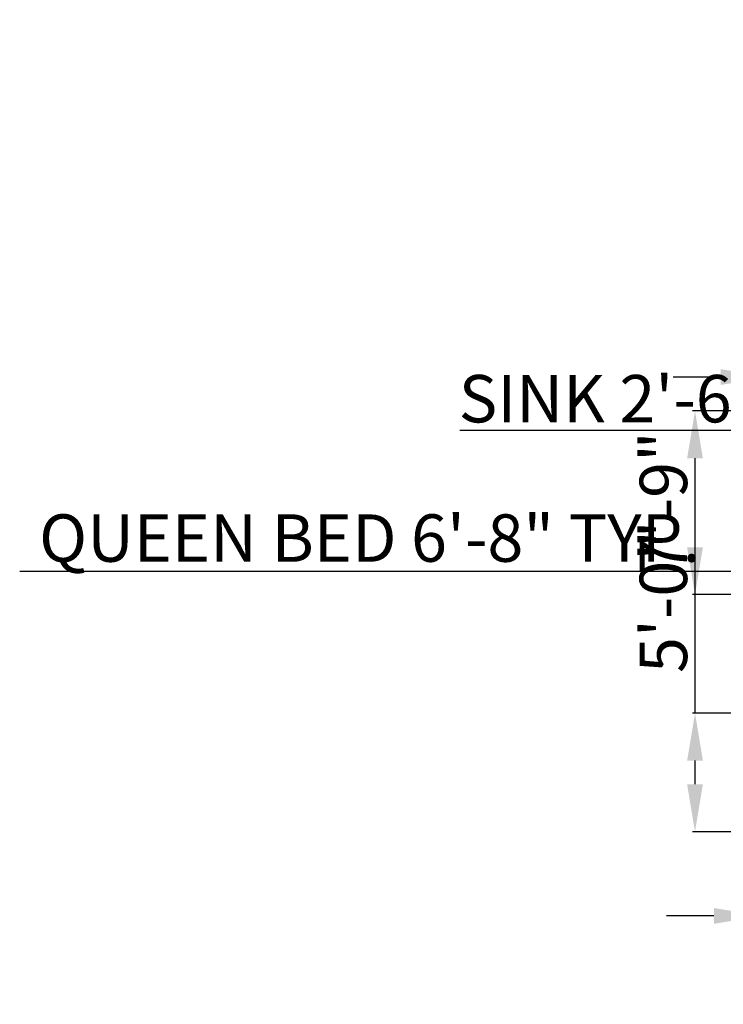
# Model space of a CAD drawing. Units: inches. Extents: x -584 to 444, y 228 to 1001.
# Tile 1 of 5: x -584 to -228, y 298 to 797. Entities that reach past the tile are written whole.
import ezdxf

# ---------------------------------------------------------------- set-up
doc = ezdxf.new("R2010")
doc.units = ezdxf.units.IN
doc.layers.add('A-ANNO-DIMS', color=2, linetype='Continuous', lineweight=18)
doc.styles.get("Standard").update_dxf_attribs({"font": 'arial.ttf'})
doc.dimstyles.new('ISO-25', dxfattribs={"dimtxt": 24, "dimasz": 24, "dimexe": 1.25, "dimexo": 0.625, "dimtad": 1, "dimdec": 1, "dimlunit": 3, "dimtxsty": 'Standard', "dimcen": 2.5, "dimadec": 0, "dimazin": 0, "dimtfac": 1, "dimtdec": 1, "dimtmove": 0, "dimatfit": 3, "dimfxl": 1, "dimarcsym": 0})

# ---------------------------------------------------------------- blocks, each defined once
blk = doc.blocks.new('*D15')
at = {"layer": 'A-ANNO-DIMS', "color": 0, "lineweight": -2, "transparency": 16777216}
for p, q in [((-206.06, 505.93), (-206.06, 518.55)), ((-126.06, 505.93), (-126.06, 518.55)), ((-206.06, 517.3), (-584.35, 517.3)), ((-150.06, 517.3), (-182.06, 517.3))]:
    blk.add_line(p, q, dxfattribs=at)
at = {"layer": 'A-ANNO-DIMS', "color": 0, "transparency": 16777216}
for points in [[(-182.06, 521.3), (-182.06, 513.3), (-206.06, 517.3)], [(-150.06, 521.3), (-150.06, 513.3), (-126.06, 517.3)]]:
    blk.add_solid(points, dxfattribs=at)
at = {"layer": 'Defpoints', "color": 0, "transparency": 16777216}
for p in [(-206.06, 517.3), (-206.06, 505.3), (-126.06, 505.3)]:
    blk.add_point(p, dxfattribs=at)
at = {"layer": 'A-ANNO-DIMS', "color": 0, "transparency": 16777216, "insert": (-407.21, 531.07), "char_height": 24, "attachment_point": 5}
blk.add_mtext('QUEEN BED 6\'-8" TYP.', dxfattribs=at)
blk = doc.blocks.new('*D19')
at = {"layer": 'A-ANNO-DIMS', "color": 0, "lineweight": -2, "transparency": 16777216}
for p, q in [((-185.21, 588.56), (-361.72, 588.56)), ((-161.21, 584.69), (-161.21, 589.81)), ((-131.21, 588.56), (-161.21, 588.56)), ((-131.21, 584.69), (-131.21, 589.81)), ((-107.21, 588.56), (-83.21, 588.56))]:
    blk.add_line(p, q, dxfattribs=at)
at = {"layer": 'A-ANNO-DIMS', "color": 0, "transparency": 16777216}
for points in [[(-185.21, 592.56), (-185.21, 584.56), (-161.21, 588.56)], [(-107.21, 592.56), (-107.21, 584.56), (-131.21, 588.56)]]:
    blk.add_solid(points, dxfattribs=at)
at = {"layer": 'Defpoints', "color": 0, "transparency": 16777216}
for p in [(-161.21, 588.56), (-161.21, 584.06), (-131.21, 584.06)]:
    blk.add_point(p, dxfattribs=at)
at = {"layer": 'A-ANNO-DIMS', "color": 0, "transparency": 16777216, "insert": (-285.47, 601.6), "char_height": 24, "attachment_point": 5}
blk.add_mtext('SINK 2\'-6"', dxfattribs=at)
blk = doc.blocks.new('*D21')
at = {"layer": 'A-ANNO-DIMS', "color": 0, "lineweight": -2, "transparency": 16777216}
for p, q in [((-186.99, 636.91), (-186.99, 660.91)), ((-189.13, 612.91), (-185.74, 612.91)), ((-186.99, 612.91), (-186.99, 594.47)), ((-189.13, 594.47), (-185.74, 594.47)), ((-186.99, 570.47), (-186.99, 298.2))]:
    blk.add_line(p, q, dxfattribs=at)
at = {"layer": 'A-ANNO-DIMS', "color": 0, "transparency": 16777216}
for points in [[(-190.99, 636.91), (-182.99, 636.91), (-186.99, 612.91)], [(-190.99, 570.47), (-182.99, 570.47), (-186.99, 594.47)]]:
    blk.add_solid(points, dxfattribs=at)
at = {"layer": 'Defpoints', "color": 0, "transparency": 16777216}
for p in [(-189.76, 612.91), (-189.76, 594.47), (-186.99, 594.47)]:
    blk.add_point(p, dxfattribs=at)
at = {"layer": 'A-ANNO-DIMS', "color": 0, "transparency": 16777216, "insert": (-200.02, 422.34), "char_height": 24, "attachment_point": 5, "rotation": 90}
blk.add_mtext('RANGE 1\'-6 1/2"', dxfattribs=at)
blk = doc.blocks.new('*D22')
at = {"layer": 'A-ANNO-DIMS', "color": 0, "lineweight": -2, "transparency": 16777216}
for p, q in [((-229.74, 615.68), (-253.74, 615.68)), ((-205.74, 613.54), (-205.74, 616.93)), ((-205.74, 615.68), (-189.76, 615.68)), ((-189.76, 613.54), (-189.76, 616.93)), ((-165.76, 615.68), (-78.97, 615.68))]:
    blk.add_line(p, q, dxfattribs=at)
at = {"layer": 'A-ANNO-DIMS', "color": 0, "transparency": 16777216}
for points in [[(-229.74, 619.68), (-229.74, 611.68), (-205.74, 615.68)], [(-165.76, 619.68), (-165.76, 611.68), (-189.76, 615.68)]]:
    blk.add_solid(points, dxfattribs=at)
at = {"layer": 'Defpoints', "color": 0, "transparency": 16777216}
for p in [(-189.76, 615.68), (-205.74, 612.91), (-189.76, 612.91)]:
    blk.add_point(p, dxfattribs=at)
at = {"layer": 'A-ANNO-DIMS', "color": 0, "transparency": 16777216, "insert": (-110.36, 628.35), "char_height": 24, "attachment_point": 5}
blk.add_mtext('1\'-4"', dxfattribs=at)
blk = doc.blocks.new('*D29')
at = {"layer": 'A-ANNO-DIMS', "color": 0, "lineweight": -2, "transparency": 16777216}
for p, q in [((-209.14, 795.91), (-209.14, 341.69)), ((-176.14, 795.91), (-176.14, 341.69)), ((-233.14, 342.94), (-257.14, 342.94)), ((-209.14, 342.94), (-176.14, 342.94)), ((-152.14, 342.94), (-62.69, 342.94))]:
    blk.add_line(p, q, dxfattribs=at)
at = {"layer": 'A-ANNO-DIMS', "color": 0, "transparency": 16777216}
for points in [[(-233.14, 346.94), (-233.14, 338.94), (-209.14, 342.94)], [(-152.14, 346.94), (-152.14, 338.94), (-176.14, 342.94)]]:
    blk.add_solid(points, dxfattribs=at)
at = {"layer": 'Defpoints', "color": 0, "transparency": 16777216}
for p in [(-209.14, 796.54), (-176.14, 796.54), (-176.14, 342.94)]:
    blk.add_point(p, dxfattribs=at)
at = {"layer": 'A-ANNO-DIMS', "color": 0, "transparency": 16777216, "insert": (-95.41, 355.82), "char_height": 24, "attachment_point": 5}
blk.add_mtext('2\'-9"', dxfattribs=at)
blk = doc.blocks.new('*D33')
at = {"layer": 'A-ANNO-DIMS', "color": 0, "lineweight": -2, "transparency": 16777216}
for p, q in [((-242.74, 445.54), (-242.74, 534.59)), ((-218.77, 445.54), (-243.99, 445.54)), ((-242.74, 409.54), (-242.74, 421.54)), ((-218.77, 385.54), (-243.99, 385.54))]:
    blk.add_line(p, q, dxfattribs=at)
at = {"layer": 'A-ANNO-DIMS', "color": 0, "transparency": 16777216}
for points in [[(-246.74, 421.54), (-238.74, 421.54), (-242.74, 445.54)], [(-246.74, 409.54), (-238.74, 409.54), (-242.74, 385.54)]]:
    blk.add_solid(points, dxfattribs=at)
at = {"layer": 'Defpoints', "color": 0, "transparency": 16777216}
for p in [(-242.74, 445.54), (-218.14, 445.54), (-218.14, 385.54)]:
    blk.add_point(p, dxfattribs=at)
at = {"layer": 'A-ANNO-DIMS', "color": 0, "transparency": 16777216, "insert": (-255.62, 502.06), "char_height": 24, "attachment_point": 5, "rotation": 90}
blk.add_mtext('5\'-0"', dxfattribs=at)
blk = doc.blocks.new('*D34')
at = {"layer": 'A-ANNO-DIMS', "color": 0, "lineweight": -2, "transparency": 16777216}
for p, q in [((-218.77, 598.54), (-243.99, 598.54)), ((-242.74, 529.54), (-242.74, 574.54)), ((-218.77, 505.54), (-243.99, 505.54))]:
    blk.add_line(p, q, dxfattribs=at)
at = {"layer": 'A-ANNO-DIMS', "color": 0, "transparency": 16777216}
for points in [[(-246.74, 574.54), (-238.74, 574.54), (-242.74, 598.54)], [(-246.74, 529.54), (-238.74, 529.54), (-242.74, 505.54)]]:
    blk.add_solid(points, dxfattribs=at)
at = {"layer": 'Defpoints', "color": 0, "transparency": 16777216}
for p in [(-242.74, 598.54), (-218.14, 598.54), (-218.14, 505.54)]:
    blk.add_point(p, dxfattribs=at)
at = {"layer": 'A-ANNO-DIMS', "color": 0, "transparency": 16777216, "insert": (-255.62, 552.04), "char_height": 24, "attachment_point": 5, "rotation": 90}
blk.add_mtext('7\'-9"', dxfattribs=at)
blk = doc.blocks.new('*D39')
at = {"layer": 'A-ANNO-DIMS', "color": 0, "lineweight": -2, "transparency": 16777216}
for p, q in [((-209.14, 645.91), (-209.14, 341.69)), ((-185.14, 645.91), (-185.14, 341.69)), ((-233.14, 342.94), (-257.14, 342.94)), ((-209.14, 342.94), (-185.14, 342.94)), ((-161.14, 342.94), (-71.69, 342.94))]:
    blk.add_line(p, q, dxfattribs=at)
at = {"layer": 'A-ANNO-DIMS', "color": 0, "transparency": 16777216}
for points in [[(-233.14, 346.94), (-233.14, 338.94), (-209.14, 342.94)], [(-161.14, 346.94), (-161.14, 338.94), (-185.14, 342.94)]]:
    blk.add_solid(points, dxfattribs=at)
at = {"layer": 'Defpoints', "color": 0, "transparency": 16777216}
for p in [(-209.14, 646.54), (-185.14, 646.54), (-185.14, 342.94)]:
    blk.add_point(p, dxfattribs=at)
at = {"layer": 'A-ANNO-DIMS', "color": 0, "transparency": 16777216, "insert": (-104.41, 355.82), "char_height": 24, "attachment_point": 5}
blk.add_mtext('2\'-0"', dxfattribs=at)

msp = doc.modelspace()

# ---------------------------------------------------------------- dimensions: what is measured, and where the dimension line sits
at = {"layer": 'A-ANNO-DIMS'}
for base, p1, p2, picture, middle in [((-176.14, 342.94), (-209.14, 796.54), (-176.14, 796.54), '*D29', (-95.41, 355.82)), ((-185.14, 342.94), (-209.14, 646.54), (-185.14, 646.54), '*D39', (-104.41, 355.82)), ((-189.76, 615.68), (-205.74, 612.91), (-189.76, 612.91), '*D22', (-110.36, 628.35))]:
    dim = msp.add_linear_dim(base=base, p1=p1, p2=p2, dimstyle='ISO-25', override={"dimdec": 1, "dimlfac": 1, "dimrnd": 0, "dimzin": 1, "dimdsep": 46, "dimlunit": 4, "dimfrac": 2}, dxfattribs=at)
    dim.commit()
    dim.dimension.update_dxf_attribs({"geometry": picture, "text_midpoint": middle})
for base, p1, p2, angle, text, picture, middle in [((-186.99, 594.47), (-189.76, 612.91), (-189.76, 594.47), 270, 'RANGE <>', '*D21', (-200.02, 422.34)), ((-161.21, 588.56), (-131.21, 584.06), (-161.21, 584.06), 180, 'SINK <>', '*D19', (-285.47, 601.6)), ((-206.06, 517.3), (-126.06, 505.3), (-206.06, 505.3), 180, 'QUEEN BED <> TYP.', '*D15', (-407.21, 531.07))]:
    dim = msp.add_linear_dim(base=base, p1=p1, p2=p2, angle=angle, text=text, dimstyle='ISO-25', override={"dimdec": 1, "dimlfac": 1, "dimrnd": 0, "dimzin": 1, "dimdsep": 46, "dimlunit": 4, "dimfrac": 2}, dxfattribs=at)
    dim.commit()
    dim.dimension.update_dxf_attribs({"geometry": picture, "text_midpoint": middle})
for base, p1, p2, picture, middle in [((-242.74, 598.54), (-218.14, 505.54), (-218.14, 598.54), '*D34', (-255.62, 552.04)), ((-242.74, 445.54), (-218.14, 385.54), (-218.14, 445.54), '*D33', (-255.62, 502.06))]:
    dim = msp.add_linear_dim(base=base, p1=p1, p2=p2, angle=90, dimstyle='ISO-25', override={"dimdec": 1, "dimlfac": 1, "dimrnd": 0, "dimzin": 1, "dimdsep": 46, "dimlunit": 4, "dimfrac": 2}, dxfattribs=at)
    dim.commit()
    dim.dimension.update_dxf_attribs({"geometry": picture, "text_midpoint": middle})

doc.saveas('drawing.dxf')
